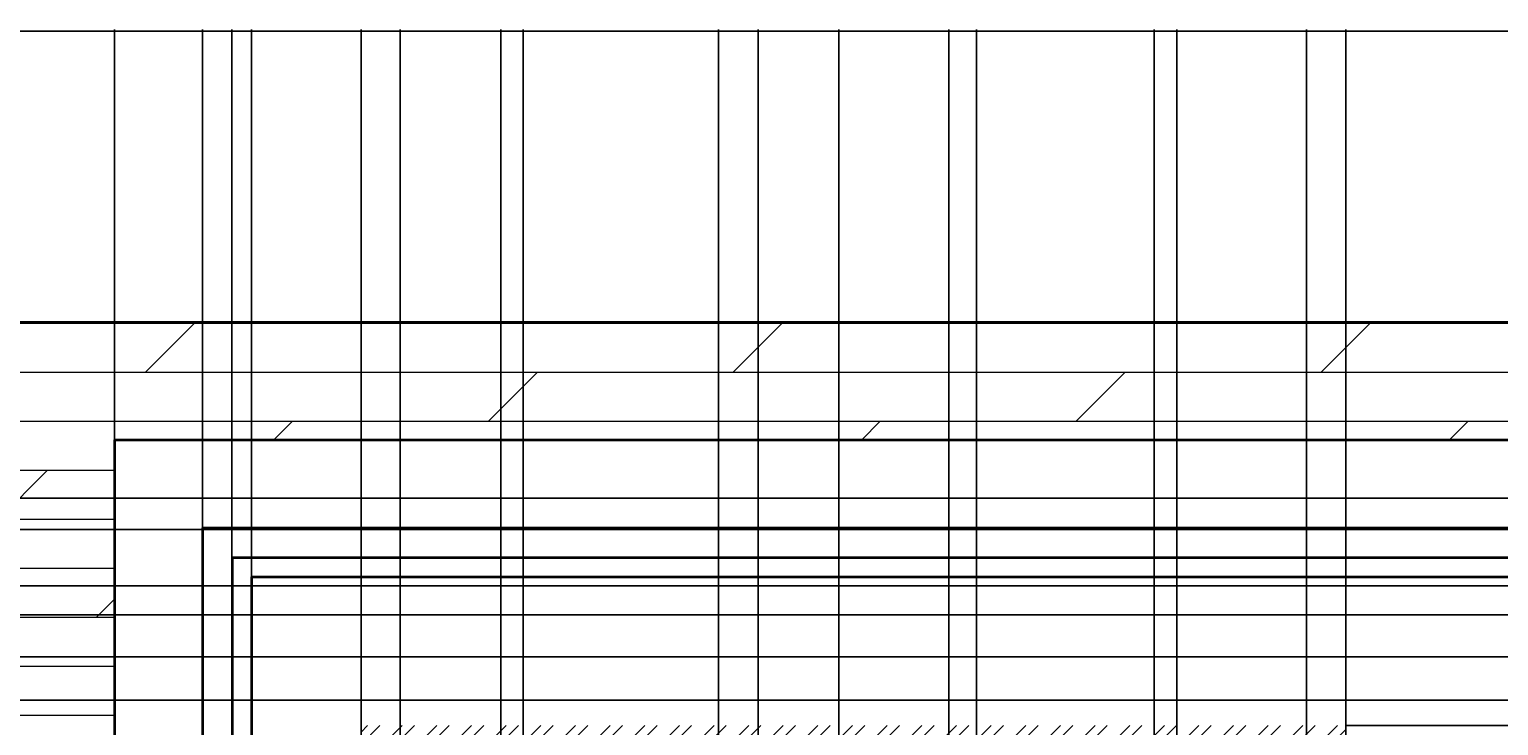
# Model space of a CAD drawing. Units: inches. Extents: x -13 to 630, y -103 to 275.
# Tile 7 of 9: x 168 to 318, y 204 to 275. Entities that reach past the tile are written whole.
import ezdxf

# ---------------------------------------------------------------- set-up
doc = ezdxf.new("R2010")
doc.units = ezdxf.units.IN
doc.header["$MEASUREMENT"] = 0
for name, color, linetype, lineweight in [('A-ANNO-DIMS', 2, 'Continuous', 18), ('A-ELEV', 7, 'Continuous', 35), ('A-ELEV-PATT', 8, 'Continuous', 13)]:
    doc.layers.add(name, color=color, linetype=linetype, lineweight=lineweight)
doc.styles.get("Standard").update_dxf_attribs({"font": 'arial.ttf'})
doc.dimstyles.get("Standard").update_dxf_attribs({"dimtxt": 0.18, "dimasz": 0.18, "dimexe": 0.18, "dimexo": 0.0625, "dimgap": 0.09, "dimtad": 0, "dimtih": 1, "dimtoh": 1, "dimdec": 4, "dimzin": 0, "dimdsep": 46, "dimtxsty": 'Standard', "dimcen": 0.09, "dimadec": 0, "dimazin": 0, "dimtfac": 1, "dimtdec": 4, "dimtofl": 0, "dimtmove": 0, "dimatfit": 3, "dimfxl": 1, "dimtolj": 1, "dimtzin": 0, "dimarcsym": 0})

# ---------------------------------------------------------------- blocks, each defined once
blk = doc.blocks.new('*D27')
at = {"layer": 'A-ANNO-DIMS', "color": 0, "lineweight": -2, "transparency": 16777216}
for p, q in [((164.84, 245.14), (164.84, 275.01)), ((165.02, 274.83), (254.62, 274.83)), ((345.13, 274.83), (255.53, 274.83)), ((345.31, 245.14), (345.31, 275.01))]:
    blk.add_line(p, q, dxfattribs=at)
at = {"layer": 'A-ANNO-DIMS', "color": 0, "transparency": 16777216}
for points in [[(165.02, 274.86), (165.02, 274.8), (164.84, 274.83)], [(345.13, 274.86), (345.13, 274.8), (345.31, 274.83)]]:
    blk.add_solid(points, dxfattribs=at)
at = {"layer": 'Defpoints', "color": 0, "transparency": 16777216}
for p in [(345.31, 274.83), (164.84, 245.08), (345.31, 245.08)]:
    blk.add_point(p, dxfattribs=at)
at = {"layer": 'A-ANNO-DIMS', "color": 0, "transparency": 16777216, "insert": (255.08, 274.83), "char_height": 0.18, "attachment_point": 5}
blk.add_mtext('\\A1;180.46', dxfattribs=at)
blk = doc.blocks.new('*D29')
at = {"layer": 'A-ANNO-DIMS', "color": 0, "lineweight": -2, "transparency": 16777216}
for p, q in [((302.59, 203.94), (630.03, 203.94)), ((629.85, 203.76), (629.85, 166.48)), ((629.85, 128.84), (629.85, 166.11)), ((302.59, 128.66), (630.03, 128.66))]:
    blk.add_line(p, q, dxfattribs=at)
at = {"layer": 'A-ANNO-DIMS', "color": 0, "transparency": 16777216}
for points in [[(629.82, 203.76), (629.88, 203.76), (629.85, 203.94)], [(629.82, 128.84), (629.88, 128.84), (629.85, 128.66)]]:
    blk.add_solid(points, dxfattribs=at)
at = {"layer": 'Defpoints', "color": 0, "transparency": 16777216}
for p in [(302.53, 203.94), (629.85, 203.94), (302.53, 128.66)]:
    blk.add_point(p, dxfattribs=at)
at = {"layer": 'A-ANNO-DIMS', "color": 0, "transparency": 16777216, "insert": (629.85, 166.3), "char_height": 0.18, "attachment_point": 5}
blk.add_mtext('\\A1;75.28', dxfattribs=at)
blk = doc.blocks.new('*D30')
at = {"layer": 'A-ANNO-DIMS', "color": 0, "lineweight": -2, "transparency": 16777216}
for p, q in [((164.84, 245.14), (164.84, 275.01)), ((165.02, 274.83), (170.63, 274.83)), ((176.66, 274.83), (171.05, 274.83)), ((176.84, 233.14), (176.84, 275.01))]:
    blk.add_line(p, q, dxfattribs=at)
at = {"layer": 'A-ANNO-DIMS', "color": 0, "transparency": 16777216}
for points in [[(165.02, 274.86), (165.02, 274.8), (164.84, 274.83)], [(176.66, 274.86), (176.66, 274.8), (176.84, 274.83)]]:
    blk.add_solid(points, dxfattribs=at)
at = {"layer": 'Defpoints', "color": 0, "transparency": 16777216}
for p in [(176.84, 274.83), (164.84, 245.08), (176.84, 233.08)]:
    blk.add_point(p, dxfattribs=at)
at = {"layer": 'A-ANNO-DIMS', "color": 0, "transparency": 16777216, "insert": (170.84, 274.83), "char_height": 0.18, "attachment_point": 5}
blk.add_mtext('\\A1;12', dxfattribs=at)
blk = doc.blocks.new('*D31')
at = {"layer": 'A-ANNO-DIMS', "color": 0, "lineweight": -2, "transparency": 16777216}
for p, q in [((176.84, 233.14), (176.84, 275.01)), ((177.02, 274.83), (181.2, 274.83)), ((185.66, 274.83), (181.49, 274.83)), ((185.84, 224.14), (185.84, 275.01))]:
    blk.add_line(p, q, dxfattribs=at)
at = {"layer": 'A-ANNO-DIMS', "color": 0, "transparency": 16777216}
for points in [[(177.02, 274.86), (177.02, 274.8), (176.84, 274.83)], [(185.66, 274.86), (185.66, 274.8), (185.84, 274.83)]]:
    blk.add_solid(points, dxfattribs=at)
at = {"layer": 'Defpoints', "color": 0, "transparency": 16777216}
for p in [(185.84, 274.83), (176.84, 233.08), (185.84, 224.08)]:
    blk.add_point(p, dxfattribs=at)
at = {"layer": 'A-ANNO-DIMS', "color": 0, "transparency": 16777216, "insert": (181.34, 274.83), "char_height": 0.18, "attachment_point": 5}
blk.add_mtext('\\A1;9', dxfattribs=at)
blk = doc.blocks.new('*D32')
at = {"layer": 'A-ANNO-DIMS', "color": 0, "lineweight": -2, "transparency": 16777216}
for p, q in [((185.84, 224.14), (185.84, 275.01)), ((186.02, 274.83), (187.2, 274.83)), ((188.66, 274.83), (187.49, 274.83)), ((188.84, 221.14), (188.84, 275.01))]:
    blk.add_line(p, q, dxfattribs=at)
at = {"layer": 'A-ANNO-DIMS', "color": 0, "transparency": 16777216}
for points in [[(186.02, 274.86), (186.02, 274.8), (185.84, 274.83)], [(188.66, 274.86), (188.66, 274.8), (188.84, 274.83)]]:
    blk.add_solid(points, dxfattribs=at)
at = {"layer": 'Defpoints', "color": 0, "transparency": 16777216}
for p in [(188.84, 274.83), (185.84, 224.08), (188.84, 221.08)]:
    blk.add_point(p, dxfattribs=at)
at = {"layer": 'A-ANNO-DIMS', "color": 0, "transparency": 16777216, "insert": (187.34, 274.83), "char_height": 0.18, "attachment_point": 5}
blk.add_mtext('\\A1;3', dxfattribs=at)
blk = doc.blocks.new('*D33')
at = {"layer": 'A-ANNO-DIMS', "color": 0, "lineweight": -2, "transparency": 16777216}
for p, q in [((188.84, 221.14), (188.84, 275.01)), ((189.02, 274.83), (189.69, 274.83)), ((190.66, 274.83), (189.99, 274.83)), ((190.84, 219.14), (190.84, 275.01))]:
    blk.add_line(p, q, dxfattribs=at)
at = {"layer": 'A-ANNO-DIMS', "color": 0, "transparency": 16777216}
for points in [[(189.02, 274.86), (189.02, 274.8), (188.84, 274.83)], [(190.66, 274.86), (190.66, 274.8), (190.84, 274.83)]]:
    blk.add_solid(points, dxfattribs=at)
at = {"layer": 'Defpoints', "color": 0, "transparency": 16777216}
for p in [(190.84, 274.83), (188.84, 221.08), (190.84, 219.08)]:
    blk.add_point(p, dxfattribs=at)
at = {"layer": 'A-ANNO-DIMS', "color": 0, "transparency": 16777216, "insert": (189.84, 274.83), "char_height": 0.18, "attachment_point": 5}
blk.add_mtext('\\A1;2', dxfattribs=at)
blk = doc.blocks.new('*D34')
at = {"layer": 'A-ANNO-DIMS', "color": 0, "lineweight": -2, "transparency": 16777216}
for p, q in [((190.84, 219.14), (190.84, 275.01)), ((191.02, 274.83), (195.98, 274.83)), ((201.84, 274.83), (196.89, 274.83)), ((202.02, 204), (202.02, 275.01))]:
    blk.add_line(p, q, dxfattribs=at)
at = {"layer": 'A-ANNO-DIMS', "color": 0, "transparency": 16777216}
for points in [[(191.02, 274.86), (191.02, 274.8), (190.84, 274.83)], [(201.84, 274.86), (201.84, 274.8), (202.02, 274.83)]]:
    blk.add_solid(points, dxfattribs=at)
at = {"layer": 'Defpoints', "color": 0, "transparency": 16777216}
for p in [(202.02, 274.83), (190.84, 219.08), (202.02, 203.94)]:
    blk.add_point(p, dxfattribs=at)
at = {"layer": 'A-ANNO-DIMS', "color": 0, "transparency": 16777216, "insert": (196.43, 274.83), "char_height": 0.18, "attachment_point": 5}
blk.add_mtext('\\A1;11.176', dxfattribs=at)
blk = doc.blocks.new('*D35')
at = {"layer": 'A-ANNO-DIMS', "color": 0, "lineweight": -2, "transparency": 16777216}
for p, q in [((319.37, 219.08), (630.03, 219.08)), ((629.85, 218.9), (629.85, 211.69)), ((629.85, 204.12), (629.85, 211.33)), ((302.59, 203.94), (630.03, 203.94))]:
    blk.add_line(p, q, dxfattribs=at)
at = {"layer": 'A-ANNO-DIMS', "color": 0, "transparency": 16777216}
for points in [[(629.82, 218.9), (629.88, 218.9), (629.85, 219.08)], [(629.82, 204.12), (629.88, 204.12), (629.85, 203.94)]]:
    blk.add_solid(points, dxfattribs=at)
at = {"layer": 'Defpoints', "color": 0, "transparency": 16777216}
for p in [(319.31, 219.08), (629.85, 219.08), (302.53, 203.94)]:
    blk.add_point(p, dxfattribs=at)
at = {"layer": 'A-ANNO-DIMS', "color": 0, "transparency": 16777216, "insert": (629.85, 211.51), "char_height": 0.18, "attachment_point": 5}
blk.add_mtext('\\A1;15.145', dxfattribs=at)
blk = doc.blocks.new('*D56')
at = {"layer": 'A-ANNO-DIMS', "color": 0, "lineweight": -2, "transparency": 16777216}
for p, q in [((206.02, 102.14), (206.02, 275.01)), ((206.2, 274.83), (210.69, 274.83)), ((216.09, 274.83), (211.6, 274.83)), ((216.27, 102.14), (216.27, 275.01))]:
    blk.add_line(p, q, dxfattribs=at)
at = {"layer": 'A-ANNO-DIMS', "color": 0, "transparency": 16777216}
for points in [[(206.2, 274.86), (206.2, 274.8), (206.02, 274.83)], [(216.09, 274.86), (216.09, 274.8), (216.27, 274.83)]]:
    blk.add_solid(points, dxfattribs=at)
at = {"layer": 'Defpoints', "color": 0, "transparency": 16777216}
for p in [(216.27, 274.83), (206.02, 102.08), (216.27, 102.08)]:
    blk.add_point(p, dxfattribs=at)
at = {"layer": 'A-ANNO-DIMS', "color": 0, "transparency": 16777216, "insert": (211.14, 274.83), "char_height": 0.18, "attachment_point": 5}
blk.add_mtext('\\A1;10.246', dxfattribs=at)
blk = doc.blocks.new('*D57')
at = {"layer": 'A-ANNO-DIMS', "color": 0, "lineweight": -2, "transparency": 16777216}
for p, q in [((216.27, 102.14), (216.27, 275.01)), ((216.45, 274.83), (217.02, 274.83)), ((218.38, 274.83), (217.81, 274.83)), ((218.56, 102.14), (218.56, 275.01))]:
    blk.add_line(p, q, dxfattribs=at)
at = {"layer": 'A-ANNO-DIMS', "color": 0, "transparency": 16777216}
for points in [[(216.45, 274.86), (216.45, 274.8), (216.27, 274.83)], [(218.38, 274.86), (218.38, 274.8), (218.56, 274.83)]]:
    blk.add_solid(points, dxfattribs=at)
at = {"layer": 'Defpoints', "color": 0, "transparency": 16777216}
for p in [(218.56, 274.83), (216.27, 102.08), (218.56, 102.08)]:
    blk.add_point(p, dxfattribs=at)
at = {"layer": 'A-ANNO-DIMS', "color": 0, "transparency": 16777216, "insert": (217.42, 274.83), "char_height": 0.18, "attachment_point": 5}
blk.add_mtext('\\A1;2.298', dxfattribs=at)
blk = doc.blocks.new('*D58')
at = {"layer": 'A-ANNO-DIMS', "color": 0, "lineweight": -2, "transparency": 16777216}
for p, q in [((218.56, 102.14), (218.56, 275.01)), ((218.74, 274.83), (228.14, 274.83)), ((238.31, 274.83), (228.91, 274.83)), ((238.49, 102.14), (238.49, 275.01))]:
    blk.add_line(p, q, dxfattribs=at)
at = {"layer": 'A-ANNO-DIMS', "color": 0, "transparency": 16777216}
for points in [[(218.74, 274.86), (218.74, 274.8), (218.56, 274.83)], [(238.31, 274.86), (238.31, 274.8), (238.49, 274.83)]]:
    blk.add_solid(points, dxfattribs=at)
at = {"layer": 'Defpoints', "color": 0, "transparency": 16777216}
for p in [(238.49, 274.83), (218.56, 102.08), (238.49, 102.08)]:
    blk.add_point(p, dxfattribs=at)
at = {"layer": 'A-ANNO-DIMS', "color": 0, "transparency": 16777216, "insert": (228.53, 274.83), "char_height": 0.18, "attachment_point": 5}
blk.add_mtext('\\A1;19.93', dxfattribs=at)
blk = doc.blocks.new('*D59')
at = {"layer": 'A-ANNO-DIMS', "color": 0, "lineweight": -2, "transparency": 16777216}
for p, q in [((238.49, 102.14), (238.49, 275.01)), ((238.67, 274.83), (251.26, 274.83)), ((264.64, 274.83), (252.05, 274.83)), ((264.82, 102.14), (264.82, 275.01))]:
    blk.add_line(p, q, dxfattribs=at)
at = {"layer": 'A-ANNO-DIMS', "color": 0, "transparency": 16777216}
for points in [[(238.67, 274.86), (238.67, 274.8), (238.49, 274.83)], [(264.64, 274.86), (264.64, 274.8), (264.82, 274.83)]]:
    blk.add_solid(points, dxfattribs=at)
at = {"layer": 'Defpoints', "color": 0, "transparency": 16777216}
for p in [(264.82, 274.83), (238.49, 102.08), (264.82, 102.08)]:
    blk.add_point(p, dxfattribs=at)
at = {"layer": 'A-ANNO-DIMS', "color": 0, "transparency": 16777216, "insert": (251.66, 274.83), "char_height": 0.18, "attachment_point": 5}
blk.add_mtext('\\A1;26.32', dxfattribs=at)
blk = doc.blocks.new('*D60')
at = {"layer": 'A-ANNO-DIMS', "color": 0, "lineweight": -2, "transparency": 16777216}
for p, q in [((264.82, 102.14), (264.82, 275.01)), ((265, 274.83), (273.44, 274.83)), ((282.8, 274.83), (274.35, 274.83)), ((282.98, 102.14), (282.98, 275.01))]:
    blk.add_line(p, q, dxfattribs=at)
at = {"layer": 'A-ANNO-DIMS', "color": 0, "transparency": 16777216}
for points in [[(265, 274.86), (265, 274.8), (264.82, 274.83)], [(282.8, 274.86), (282.8, 274.8), (282.98, 274.83)]]:
    blk.add_solid(points, dxfattribs=at)
at = {"layer": 'Defpoints', "color": 0, "transparency": 16777216}
for p in [(282.98, 274.83), (264.82, 102.08), (282.98, 102.08)]:
    blk.add_point(p, dxfattribs=at)
at = {"layer": 'A-ANNO-DIMS', "color": 0, "transparency": 16777216, "insert": (273.9, 274.83), "char_height": 0.18, "attachment_point": 5}
blk.add_mtext('\\A1;18.158', dxfattribs=at)
blk = doc.blocks.new('*D61')
at = {"layer": 'A-ANNO-DIMS', "color": 0, "lineweight": -2, "transparency": 16777216}
for p, q in [((282.98, 102.14), (282.98, 275.01)), ((283.16, 274.83), (283.73, 274.83)), ((285.09, 274.83), (284.52, 274.83)), ((285.27, 102.14), (285.27, 275.01))]:
    blk.add_line(p, q, dxfattribs=at)
at = {"layer": 'A-ANNO-DIMS', "color": 0, "transparency": 16777216}
for points in [[(283.16, 274.86), (283.16, 274.8), (282.98, 274.83)], [(285.09, 274.86), (285.09, 274.8), (285.27, 274.83)]]:
    blk.add_solid(points, dxfattribs=at)
at = {"layer": 'Defpoints', "color": 0, "transparency": 16777216}
for p in [(285.27, 274.83), (282.98, 102.08), (285.27, 102.08)]:
    blk.add_point(p, dxfattribs=at)
at = {"layer": 'A-ANNO-DIMS', "color": 0, "transparency": 16777216, "insert": (284.12, 274.83), "char_height": 0.18, "attachment_point": 5}
blk.add_mtext('\\A1;2.298', dxfattribs=at)
blk = doc.blocks.new('*D62')
at = {"layer": 'A-ANNO-DIMS', "color": 0, "lineweight": -2, "transparency": 16777216}
for p, q in [((285.27, 102.14), (285.27, 275.01)), ((285.45, 274.83), (291.44, 274.83)), ((298.35, 274.83), (292.35, 274.83)), ((298.53, 102.14), (298.53, 275.01))]:
    blk.add_line(p, q, dxfattribs=at)
at = {"layer": 'A-ANNO-DIMS', "color": 0, "transparency": 16777216}
for points in [[(285.45, 274.86), (285.45, 274.8), (285.27, 274.83)], [(298.35, 274.86), (298.35, 274.8), (298.53, 274.83)]]:
    blk.add_solid(points, dxfattribs=at)
at = {"layer": 'Defpoints', "color": 0, "transparency": 16777216}
for p in [(298.53, 274.83), (285.27, 102.08), (298.53, 102.08)]:
    blk.add_point(p, dxfattribs=at)
at = {"layer": 'A-ANNO-DIMS', "color": 0, "transparency": 16777216, "insert": (291.9, 274.83), "char_height": 0.18, "attachment_point": 5}
blk.add_mtext('\\A1;13.253', dxfattribs=at)
blk = doc.blocks.new('*D63')
at = {"layer": 'A-ANNO-DIMS', "color": 0, "lineweight": -2, "transparency": 16777216}
for p, q in [((202.02, 128.72), (202.02, 275.01)), ((202.2, 274.83), (221.81, 274.83)), ((242.35, 274.83), (222.74, 274.83)), ((242.53, 128.72), (242.53, 275.01))]:
    blk.add_line(p, q, dxfattribs=at)
at = {"layer": 'A-ANNO-DIMS', "color": 0, "transparency": 16777216}
for points in [[(202.2, 274.86), (202.2, 274.8), (202.02, 274.83)], [(242.35, 274.86), (242.35, 274.8), (242.53, 274.83)]]:
    blk.add_solid(points, dxfattribs=at)
at = {"layer": 'Defpoints', "color": 0, "transparency": 16777216}
for p in [(242.53, 274.83), (202.02, 128.66), (242.53, 128.66)]:
    blk.add_point(p, dxfattribs=at)
at = {"layer": 'A-ANNO-DIMS', "color": 0, "transparency": 16777216, "insert": (222.27, 274.83), "char_height": 0.18, "attachment_point": 5}
blk.add_mtext('\\A1;40.505', dxfattribs=at)
blk = doc.blocks.new('*D64')
at = {"layer": 'A-ANNO-DIMS', "color": 0, "lineweight": -2, "transparency": 16777216}
for p, q in [((242.53, 128.72), (242.53, 275.01)), ((242.71, 274.83), (246.25, 274.83)), ((250.59, 274.83), (247.04, 274.83)), ((250.77, 128.2), (250.77, 275.01))]:
    blk.add_line(p, q, dxfattribs=at)
at = {"layer": 'A-ANNO-DIMS', "color": 0, "transparency": 16777216}
for points in [[(242.71, 274.86), (242.71, 274.8), (242.53, 274.83)], [(250.59, 274.86), (250.59, 274.8), (250.77, 274.83)]]:
    blk.add_solid(points, dxfattribs=at)
at = {"layer": 'Defpoints', "color": 0, "transparency": 16777216}
for p in [(250.77, 274.83), (242.53, 128.66), (250.77, 128.14)]:
    blk.add_point(p, dxfattribs=at)
at = {"layer": 'A-ANNO-DIMS', "color": 0, "transparency": 16777216, "insert": (246.65, 274.83), "char_height": 0.18, "attachment_point": 5}
blk.add_mtext('\\A1;8.244', dxfattribs=at)
blk = doc.blocks.new('*D65')
at = {"layer": 'A-ANNO-DIMS', "color": 0, "lineweight": -2, "transparency": 16777216}
for p, q in [((250.77, 128.2), (250.77, 275.01)), ((250.95, 274.83), (256.01, 274.83)), ((261.84, 274.83), (256.78, 274.83)), ((262.02, 128.72), (262.02, 275.01))]:
    blk.add_line(p, q, dxfattribs=at)
at = {"layer": 'A-ANNO-DIMS', "color": 0, "transparency": 16777216}
for points in [[(250.95, 274.86), (250.95, 274.8), (250.77, 274.83)], [(261.84, 274.86), (261.84, 274.8), (262.02, 274.83)]]:
    blk.add_solid(points, dxfattribs=at)
at = {"layer": 'Defpoints', "color": 0, "transparency": 16777216}
for p in [(262.02, 274.83), (250.77, 128.14), (262.02, 128.66)]:
    blk.add_point(p, dxfattribs=at)
at = {"layer": 'A-ANNO-DIMS', "color": 0, "transparency": 16777216, "insert": (256.4, 274.83), "char_height": 0.18, "attachment_point": 5}
blk.add_mtext('\\A1;11.25', dxfattribs=at)
blk = doc.blocks.new('*D66')
at = {"layer": 'A-ANNO-DIMS', "color": 0, "lineweight": -2, "transparency": 16777216}
for p, q in [((262.02, 128.72), (262.02, 275.01)), ((262.2, 274.83), (281.81, 274.83)), ((302.35, 274.83), (282.74, 274.83)), ((302.53, 128.72), (302.53, 275.01))]:
    blk.add_line(p, q, dxfattribs=at)
at = {"layer": 'A-ANNO-DIMS', "color": 0, "transparency": 16777216}
for points in [[(262.2, 274.86), (262.2, 274.8), (262.02, 274.83)], [(302.35, 274.86), (302.35, 274.8), (302.53, 274.83)]]:
    blk.add_solid(points, dxfattribs=at)
at = {"layer": 'Defpoints', "color": 0, "transparency": 16777216}
for p in [(302.53, 274.83), (262.02, 128.66), (302.53, 128.66)]:
    blk.add_point(p, dxfattribs=at)
at = {"layer": 'A-ANNO-DIMS', "color": 0, "transparency": 16777216, "insert": (282.27, 274.83), "char_height": 0.18, "attachment_point": 5}
blk.add_mtext('\\A1;40.505', dxfattribs=at)
blk = doc.blocks.new('*D89')
at = {"layer": 'A-ANNO-DIMS', "color": 0, "lineweight": -2, "transparency": 16777216}
for p, q in [((95.18, 210.97), (630.03, 210.97)), ((629.85, 210.79), (629.85, 208.93)), ((629.85, 206.71), (629.85, 208.57)), ((95.18, 206.53), (630.03, 206.53))]:
    blk.add_line(p, q, dxfattribs=at)
at = {"layer": 'A-ANNO-DIMS', "color": 0, "transparency": 16777216}
for points in [[(629.82, 210.79), (629.88, 210.79), (629.85, 210.97)], [(629.82, 206.71), (629.88, 206.71), (629.85, 206.53)]]:
    blk.add_solid(points, dxfattribs=at)
at = {"layer": 'Defpoints', "color": 0, "transparency": 16777216}
for p in [(95.12, 210.97), (629.85, 210.97), (95.12, 206.53)]:
    blk.add_point(p, dxfattribs=at)
at = {"layer": 'A-ANNO-DIMS', "color": 0, "transparency": 16777216, "insert": (629.85, 208.75), "char_height": 0.18, "attachment_point": 5}
blk.add_mtext('\\A1;4.442', dxfattribs=at)
blk = doc.blocks.new('*D90')
at = {"layer": 'A-ANNO-DIMS', "color": 0, "lineweight": -2, "transparency": 16777216}
for p, q in [((95.18, 218.21), (630.03, 218.21)), ((629.85, 218.03), (629.85, 214.77)), ((629.85, 211.15), (629.85, 214.41)), ((95.18, 210.97), (630.03, 210.97))]:
    blk.add_line(p, q, dxfattribs=at)
at = {"layer": 'A-ANNO-DIMS', "color": 0, "transparency": 16777216}
for points in [[(629.82, 218.03), (629.88, 218.03), (629.85, 218.21)], [(629.82, 211.15), (629.88, 211.15), (629.85, 210.97)]]:
    blk.add_solid(points, dxfattribs=at)
at = {"layer": 'Defpoints', "color": 0, "transparency": 16777216}
for p in [(95.12, 218.21), (629.85, 218.21), (95.12, 210.97)]:
    blk.add_point(p, dxfattribs=at)
at = {"layer": 'A-ANNO-DIMS', "color": 0, "transparency": 16777216, "insert": (629.85, 214.59), "char_height": 0.18, "attachment_point": 5}
blk.add_mtext('\\A1;7.236', dxfattribs=at)
blk = doc.blocks.new('*D91')
at = {"layer": 'A-ANNO-DIMS', "color": 0, "lineweight": -2, "transparency": 16777216}
for p, q in [((54.98, 218.21), (630.03, 218.21)), ((629.85, 218.03), (629.85, 216.9)), ((629.85, 215.41), (629.85, 216.54)), ((54.98, 215.23), (630.03, 215.23))]:
    blk.add_line(p, q, dxfattribs=at)
at = {"layer": 'A-ANNO-DIMS', "color": 0, "transparency": 16777216}
for points in [[(629.82, 218.03), (629.88, 218.03), (629.85, 218.21)], [(629.82, 215.41), (629.88, 215.41), (629.85, 215.23)]]:
    blk.add_solid(points, dxfattribs=at)
at = {"layer": 'Defpoints', "color": 0, "transparency": 16777216}
for p in [(54.92, 218.21), (629.85, 218.21), (54.92, 215.23)]:
    blk.add_point(p, dxfattribs=at)
at = {"layer": 'A-ANNO-DIMS', "color": 0, "transparency": 16777216, "insert": (629.85, 216.72), "char_height": 0.18, "attachment_point": 5}
blk.add_mtext('\\A1;2.972', dxfattribs=at)
blk = doc.blocks.new('*D94')
at = {"layer": 'A-ANNO-DIMS', "color": 0, "lineweight": -2, "transparency": 16777216}
for p, q in [((99.2, 227.15), (630.03, 227.15)), ((629.85, 226.97), (629.85, 225.73)), ((629.85, 224.12), (629.85, 225.36)), ((99.2, 223.94), (630.03, 223.94))]:
    blk.add_line(p, q, dxfattribs=at)
at = {"layer": 'A-ANNO-DIMS', "color": 0, "transparency": 16777216}
for points in [[(629.82, 226.97), (629.88, 226.97), (629.85, 227.15)], [(629.82, 224.12), (629.88, 224.12), (629.85, 223.94)]]:
    blk.add_solid(points, dxfattribs=at)
at = {"layer": 'Defpoints', "color": 0, "transparency": 16777216}
for p in [(99.14, 227.15), (629.85, 227.15), (99.14, 223.94)]:
    blk.add_point(p, dxfattribs=at)
at = {"layer": 'A-ANNO-DIMS', "color": 0, "transparency": 16777216, "insert": (629.85, 225.55), "char_height": 0.18, "attachment_point": 5}
blk.add_mtext('\\A1;3.21', dxfattribs=at)

msp = doc.modelspace()

# ---------------------------------------------------------------- hatches: boundary and pattern name
at = {"layer": 'A-ELEV-PATT', "transparency": 33554541}
h = msp.add_hatch(dxfattribs=at)
h.set_pattern_fill('DOLMIT', color=256, scale=20)
h.paths.add_polyline_path([(345.3061, 245.0808), (164.8443, 245.0808), (164.8443, 5.0808), (176.8443, 5.0808), (176.8443, 233.0808), (333.3061, 233.0808), (333.3061, 5.0808), (345.3061, 5.0808)])
at = {"layer": 'A-ELEV-PATT'}
h = msp.add_hatch(dxfattribs=at)
h.set_pattern_fill('BRSTONE', color=256, scale=20)
h.paths.add_polyline_path([(120.6641, 172.7854), (64.9953, 172.7854, 0.41421356), (54.9953, 162.7854), (54.9953, 125.0808), (59.9953, 125.0808), (59.9953, 162.7854, -0.41421356), (64.9953, 167.7854), (120.6641, 167.7854, -0.41421356), (125.6641, 162.7854), (125.6641, 125.0808), (130.6641, 125.0808), (130.6641, 162.7854, 0.41421356)])
h.paths.add_polyline_path([(439.5513, 172.7854), (383.8825, 172.7854, 0.41421356), (373.8825, 162.7854), (373.8825, 125.0808), (378.8825, 125.0808), (378.8825, 162.7854, -0.41421356), (383.8825, 167.7854), (439.5513, 167.7854, -0.41421356), (444.5513, 162.7854), (444.5513, 125.0808), (449.5513, 125.0808), (449.5513, 162.7854, 0.41421356)])
h.paths.add_polyline_path([(364.7117, 113.0808), (484.7117, 113.0808), (484.7117, 5.0808), (496.7117, 5.0808), (496.7117, 125.0808), (345.3061, 125.0808), (345.3061, 5.0808), (364.7117, 5.0808)])
h.paths.add_polyline_path([(164.8443, 125.0808), (28.7117, 125.0808), (16.7117, 125.0808), (16.7117, 5.0808), (28.7117, 5.0808), (28.7117, 113.0808), (148.7117, 113.0808), (148.7117, 5.0808), (164.8443, 5.0808)])
h.paths.add_polyline_path([(95.1171, 223.9392), (83.8622, 223.9392), (83.8622, 206.5279), (95.1171, 206.5279)])
h.paths.add_polyline_path([(54.9212, 223.9392), (40.7186, 223.9392), (40.7186, 206.5279), (54.9212, 206.5279)])
h.paths.add_polyline_path([(463.828, 223.9392), (449.6254, 223.9392), (449.6254, 206.5279), (463.828, 206.5279)])
h.paths.add_polyline_path([(420.6843, 223.9392), (409.4295, 223.9392), (409.4295, 206.5279), (420.6843, 206.5279)])
h = msp.add_hatch(dxfattribs=at)
h.set_pattern_fill('STEEL', color=256, scale=20)
h.set_pattern_definition([(45, (0, 0), (-1.767767, 1.767767), []), (45, (0, 1.25), (-1.767767, 1.767767), [])])
h.paths.add_polyline_path([(164.8443, 218.2056), (95.1171, 218.2056), (95.1171, 215.2335), (164.8443, 215.2335)])
h.paths.add_polyline_path([(83.8622, 218.2056), (54.9212, 218.2056), (54.9212, 215.2335), (83.8622, 215.2335)])
h.paths.add_polyline_path([(409.4295, 218.2056), (345.3061, 218.2056), (345.3061, 215.2335), (409.4295, 215.2335)])
h.paths.add_polyline_path([(449.6254, 218.2056), (420.6843, 218.2056), (420.6843, 215.2335), (449.6254, 215.2335)])
h.paths.add_polyline_path([(302.5258, 203.9359), (202.0208, 203.9359), (202.0208, 128.6551, -0.36718729), (252.2733, 187.858, -0.36718729), (302.5258, 128.6551)])

# ---------------------------------------------------------------- linework, layer by layer
at = {"layer": 'A-ELEV'}
for points in [[(345.3061, 5.0808), (345.3061, 245.0808), (164.8443, 245.0808), (164.8443, 5.0808)], [(333.3061, 5.0808), (333.3061, 233.0808), (176.8443, 233.0808), (176.8443, 5.0808)], [(324.3061, 5.0808), (324.3061, 224.0808), (185.8443, 224.0808), (185.8443, 5.0808)], [(321.3061, 5.0808), (321.3061, 221.0808), (188.8443, 221.0808), (188.8443, 5.0808)], [(319.3061, 5.0808), (319.3061, 219.0808), (190.8443, 219.0808), (190.8443, 5.0808)]]:
    msp.add_lwpolyline(points, dxfattribs=at)

# ---------------------------------------------------------------- dimensions: what is measured, and where the dimension line sits
at = {"layer": 'A-ANNO-DIMS'}
for base, p1, p2, override, picture, middle in [((345.3061, 274.8308), (164.8443, 245.0808), (345.3061, 245.0808), {"dimdec": 2, "dimlfac": 1, "dimrnd": 0, "dimzin": 0, "dimdsep": 46, "dimlunit": 2}, '*D27', (255.0752, 274.8308)), ((176.8443, 274.8308), (164.8443, 245.0808), (176.8443, 233.0808), {"dimdec": 0, "dimlfac": 1, "dimrnd": 0, "dimzin": 0, "dimdsep": 46, "dimlunit": 2}, '*D30', (170.8443, 274.8308)), ((185.8443, 274.8308), (176.8443, 233.0808), (185.8443, 224.0808), {"dimdec": 0, "dimlfac": 1, "dimrnd": 0, "dimzin": 0, "dimdsep": 46, "dimlunit": 2}, '*D31', (181.3443, 274.8308)), ((188.8443, 274.8308), (185.8443, 224.0808), (188.8443, 221.0808), {"dimdec": 0, "dimlfac": 1, "dimrnd": 0, "dimzin": 0, "dimdsep": 46, "dimlunit": 2}, '*D32', (187.3443, 274.8308)), ((190.8443, 274.8308), (188.8443, 221.0808), (190.8443, 219.0808), {"dimdec": 0, "dimlfac": 1, "dimrnd": 0, "dimzin": 0, "dimdsep": 46, "dimlunit": 2}, '*D33', (189.8443, 274.8308)), ((202.02079, 274.83079), (190.8443, 219.08079), (202.02079, 203.93592), {"dimdec": 3, "dimlfac": 1, "dimrnd": 0, "dimzin": 0, "dimdsep": 46, "dimlunit": 2}, '*D34', (196.43255, 274.83079)), ((242.5258, 274.8308), (202.0208, 128.6551), (242.5258, 128.6551), {"dimdec": 3, "dimlfac": 1, "dimrnd": 0, "dimzin": 0, "dimdsep": 46, "dimlunit": 2}, '*D63', (222.2733, 274.8308)), ((216.2667, 274.8308), (206.0208, 102.0808), (216.2667, 102.0808), {"dimdec": 3, "dimlfac": 1, "dimrnd": 0, "dimzin": 0, "dimdsep": 46, "dimlunit": 2}, '*D56', (211.1438, 274.8308)), ((218.5646, 274.8308), (216.2667, 102.0808), (218.5646, 102.0808), {"dimdec": 3, "dimlfac": 1, "dimrnd": 0, "dimzin": 0, "dimdsep": 46, "dimlunit": 2}, '*D57', (217.4157, 274.8308)), ((238.4945, 274.8308), (218.5646, 102.0808), (238.4945, 102.0808), {"dimdec": 2, "dimlfac": 1, "dimrnd": 0, "dimzin": 0, "dimdsep": 46, "dimlunit": 2}, '*D58', (228.5295, 274.8308)), ((264.8171, 274.8308), (238.4945, 102.0808), (264.8171, 102.0808), {"dimdec": 2, "dimlfac": 1, "dimrnd": 0, "dimzin": 0, "dimdsep": 46, "dimlunit": 2}, '*D59', (251.6558, 274.8308)), ((250.7699, 274.8308), (242.5258, 128.6551), (250.7699, 128.137), {"dimdec": 3, "dimlfac": 1, "dimrnd": 0, "dimzin": 0, "dimdsep": 46, "dimlunit": 2}, '*D64', (246.6478, 274.8308)), ((262.0208, 274.8308), (250.7699, 128.137), (262.0208, 128.6551), {"dimdec": 2, "dimlfac": 1, "dimrnd": 0, "dimzin": 0, "dimdsep": 46, "dimlunit": 2}, '*D65', (256.3953, 274.8308)), ((302.5258, 274.8308), (262.0208, 128.6551), (302.5258, 128.6551), {"dimdec": 3, "dimlfac": 1, "dimrnd": 0, "dimzin": 0, "dimdsep": 46, "dimlunit": 2}, '*D66', (282.2733, 274.8308)), ((282.9751, 274.8308), (264.8171, 102.0808), (282.9751, 102.0808), {"dimdec": 3, "dimlfac": 1, "dimrnd": 0, "dimzin": 0, "dimdsep": 46, "dimlunit": 2}, '*D60', (273.8961, 274.8308)), ((285.273, 274.8308), (282.9751, 102.0808), (285.273, 102.0808), {"dimdec": 3, "dimlfac": 1, "dimrnd": 0, "dimzin": 0, "dimdsep": 46, "dimlunit": 2}, '*D61', (284.1241, 274.8308)), ((298.5258, 274.8308), (285.273, 102.0808), (298.5258, 102.0808), {"dimdec": 3, "dimlfac": 1, "dimrnd": 0, "dimzin": 0, "dimdsep": 46, "dimlunit": 2}, '*D62', (291.8994, 274.8308))]:
    dim = msp.add_linear_dim(base=base, p1=p1, p2=p2, dimstyle='Standard', override=override, dxfattribs=at)
    dim.commit()
    dim.dimension.update_dxf_attribs({"geometry": picture, "text_midpoint": middle})
for base, p1, p2, override, picture, middle in [((629.8508, 227.1518), (99.1367, 223.9392), (99.1367, 227.1518), {"dimdec": 2, "dimlfac": 1, "dimrnd": 0, "dimzin": 0, "dimdsep": 46, "dimlunit": 2}, '*D94', (629.8508, 225.5455)), ((629.8508, 219.0808), (302.5258, 203.9359), (319.3061, 219.0808), {"dimdec": 3, "dimlfac": 1, "dimrnd": 0, "dimzin": 0, "dimdsep": 46, "dimlunit": 2}, '*D35', (629.8508, 211.5084)), ((629.8508, 218.2056), (54.9212, 215.2335), (54.9212, 218.2056), {"dimdec": 3, "dimlfac": 1, "dimrnd": 0, "dimzin": 0, "dimdsep": 46, "dimlunit": 2}, '*D91', (629.8508, 216.7196)), ((629.8508, 218.2056), (95.1171, 210.9698), (95.1171, 218.2056), {"dimdec": 3, "dimlfac": 1, "dimrnd": 0, "dimzin": 0, "dimdsep": 46, "dimlunit": 2}, '*D90', (629.8508, 214.5877)), ((629.8508, 210.9698), (95.1171, 206.5279), (95.1171, 210.9698), {"dimdec": 3, "dimlfac": 1, "dimrnd": 0, "dimzin": 0, "dimdsep": 46, "dimlunit": 2}, '*D89', (629.8508, 208.7489)), ((629.8508, 203.9359), (302.5258, 128.6551), (302.5258, 203.9359), {"dimdec": 2, "dimlfac": 1, "dimrnd": 0, "dimzin": 0, "dimdsep": 46, "dimlunit": 2}, '*D29', (629.8508, 166.2955))]:
    dim = msp.add_linear_dim(base=base, p1=p1, p2=p2, angle=90, dimstyle='Standard', override=override, dxfattribs=at)
    dim.commit()
    dim.dimension.update_dxf_attribs({"geometry": picture, "text_midpoint": middle})

doc.saveas('drawing.dxf')
